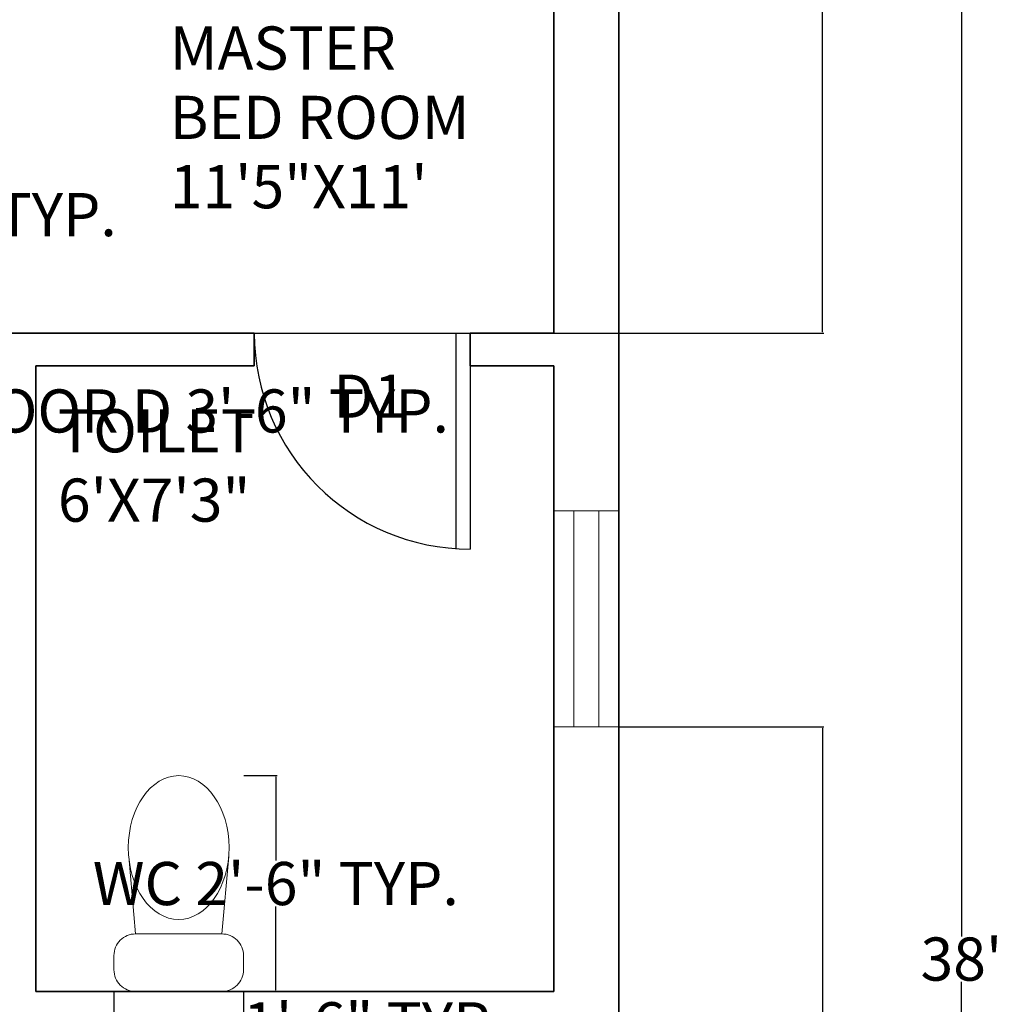
# Model space of a CAD drawing. Units: inches. Extents: x -26 to 575, y -18 to 513.
# Tile 27 of 28: x 439 to 575, y 241 to 378. Entities that reach past the tile are written whole.
import ezdxf

# ---------------------------------------------------------------- set-up
doc = ezdxf.new("R2010")
doc.units = ezdxf.units.IN
doc.header["$MEASUREMENT"] = 0
for name, color, linetype, lineweight in [('A-ANNO-DIMS', 2, 'Continuous', 18), ('A-ANNO-TEXT', 7, 'Continuous', 18), ('A-AREA-IDEN', 7, 'Continuous', 18), ('A-DOOR', 3, 'Continuous', 25), ('A-FLOR-FIXT', 9, 'Continuous', 18), ('A-GLAZ', 4, 'Continuous', 18), ('A-WALL', 7, 'Continuous', 35)]:
    doc.layers.add(name, color=color, linetype=linetype, lineweight=lineweight)
doc.styles.get("Standard").update_dxf_attribs({"font": 'arial.ttf', "height": 6})
doc.dimstyles.get("Standard").update_dxf_attribs({"dimtxt": 6, "dimasz": 0.18, "dimexe": 0.18, "dimexo": 0.0625, "dimgap": 0.09, "dimtad": 0, "dimtih": 1, "dimtoh": 1, "dimzin": 0, "dimdsep": 46, "dimlunit": 3, "dimtxsty": 'Standard', "dimcen": 0.09, "dimadec": 0, "dimazin": 0, "dimtfac": 1, "dimtofl": 0, "dimtmove": 0, "dimatfit": 3, "dimfxl": 1, "dimtolj": 1, "dimtzin": 0, "dimarcsym": 0})

# ---------------------------------------------------------------- blocks, each defined once
blk = doc.blocks.new('*D2')
at = {"layer": 'A-ANNO-DIMS', "color": 0, "lineweight": -2, "transparency": 16777216}
for p, q in [((522.24, 475.51), (569.98, 475.51)), ((569.8, 475.33), (569.8, 250.66)), ((569.8, 19.69), (569.8, 244.35)), ((522.24, 19.51), (569.98, 19.51))]:
    blk.add_line(p, q, dxfattribs=at)
at = {"layer": 'A-ANNO-DIMS', "color": 0, "transparency": 16777216}
for points in [[(569.77, 475.33), (569.83, 475.33), (569.8, 475.51)], [(569.77, 19.69), (569.83, 19.69), (569.8, 19.51)]]:
    blk.add_solid(points, dxfattribs=at)
at = {"layer": 'Defpoints', "color": 0, "transparency": 16777216}
for p in [(522.18, 475.51), (522.18, 19.51), (569.8, 19.51)]:
    blk.add_point(p, dxfattribs=at)
at = {"layer": 'A-ANNO-DIMS', "color": 0, "transparency": 16777216, "insert": (569.8, 247.51), "char_height": 6, "attachment_point": 5}
blk.add_mtext("\\A1;38'", dxfattribs=at)
blk = doc.blocks.new('DOOR-SWING-30IN')
for p, q in [((-30, 0), (0, 0)), ((-2, 0), (-2, -30)), ((0, 0), (0, -30))]:
    blk.add_line(p, q)
blk.add_arc((0, 0), 30, 180, 270)
blk = doc.blocks.new('WINDOW-30IN')
for p, q in [((30, 9), (0, 9)), ((0, 9), (0, 0)), ((30, 0), (30, 9)), ((30, 6.25), (0, 6.25)), ((30, 0), (30, 4.5)), ((30, 2.75), (0, 2.75)), ((0, 0), (30, 0))]:
    blk.add_line(p, q)
blk = doc.blocks.new('WC-FLOOR-MOUNT')
for p, q in [((-6, 8), (-6.95, 18.75)), ((6, 8), (6.95, 18.75))]:
    blk.add_line(p, q)
blk.add_lwpolyline([(-6, 8), (6, 8, -0.414214), (9, 5), (9, 3, -0.414214), (6, 0), (-6, 0, -0.414214), (-9, 3), (-9, 5, -0.414214)], format="xyb", close=True)
blk.add_ellipse((0, 20), major_axis=(0, 10), ratio=0.7)
blk = doc.blocks.new('*D14')
at = {"layer": 'A-ANNO-DIMS', "color": 0, "lineweight": -2, "transparency": 16777216}
for p, q in [((385.8, 329.95), (385.8, 323.53)), ((427.8, 329.95), (427.8, 323.53)), ((385.98, 323.71), (427.62, 323.71)), ((427.8, 323.71), (427.98, 323.71))]:
    blk.add_line(p, q, dxfattribs=at)
at = {"layer": 'A-ANNO-DIMS', "color": 0, "transparency": 16777216}
for points in [[(385.98, 323.74), (385.98, 323.68), (385.8, 323.71)], [(427.62, 323.74), (427.62, 323.68), (427.8, 323.71)]]:
    blk.add_solid(points, dxfattribs=at)
at = {"layer": 'Defpoints', "color": 0, "transparency": 16777216}
for p in [(385.8, 330.01), (427.8, 330.01), (427.8, 323.71)]:
    blk.add_point(p, dxfattribs=at)
at = {"layer": 'A-ANNO-DIMS', "color": 0, "transparency": 16777216, "insert": (464.13, 323.71), "char_height": 6, "attachment_point": 5}
blk.add_mtext('\\A1;DOOR D 3\'-6" TYP.', dxfattribs=at)
blk = doc.blocks.new('*D15')
at = {"layer": 'A-ANNO-DIMS', "color": 0, "lineweight": -2, "transparency": 16777216}
for p, q in [((427.86, 372.01), (434.28, 372.01)), ((434.1, 371.83), (434.1, 354.16)), ((434.1, 330.19), (434.1, 347.85)), ((427.86, 330.01), (434.28, 330.01))]:
    blk.add_line(p, q, dxfattribs=at)
at = {"layer": 'A-ANNO-DIMS', "color": 0, "transparency": 16777216}
for points in [[(434.07, 371.83), (434.13, 371.83), (434.1, 372.01)], [(434.07, 330.19), (434.13, 330.19), (434.1, 330.01)]]:
    blk.add_solid(points, dxfattribs=at)
at = {"layer": 'Defpoints', "color": 0, "transparency": 16777216}
for p in [(427.8, 372.01), (434.1, 372.01), (427.8, 330.01)]:
    blk.add_point(p, dxfattribs=at)
at = {"layer": 'A-ANNO-DIMS', "color": 0, "transparency": 16777216, "insert": (434.1, 351.01), "char_height": 6, "attachment_point": 5}
blk.add_mtext('\\A1;3\'-6" TYP.', dxfattribs=at)
blk = doc.blocks.new('*D20')
at = {"layer": 'A-ANNO-DIMS', "color": 0, "lineweight": -2, "transparency": 16777216}
for p, q in [((470.08, 273.01), (474.7, 273.01)), ((474.52, 272.83), (474.52, 261.2)), ((474.52, 243.19), (474.52, 254.82)), ((470.08, 243.01), (474.7, 243.01))]:
    blk.add_line(p, q, dxfattribs=at)
at = {"layer": 'A-ANNO-DIMS', "color": 0, "transparency": 16777216}
for points in [[(474.49, 272.83), (474.55, 272.83), (474.52, 273.01)], [(474.49, 243.19), (474.55, 243.19), (474.52, 243.01)]]:
    blk.add_solid(points, dxfattribs=at)
at = {"layer": 'Defpoints', "color": 0, "transparency": 16777216}
for p in [(470.02, 273.01), (474.52, 273.01), (470.02, 243.01)]:
    blk.add_point(p, dxfattribs=at)
at = {"layer": 'A-ANNO-DIMS', "color": 0, "transparency": 16777216, "insert": (474.52, 258.01), "char_height": 6, "attachment_point": 5}
blk.add_mtext('\\A1;WC 2\'-6" TYP.', dxfattribs=at)
blk = doc.blocks.new('*D21')
at = {"layer": 'A-ANNO-DIMS', "color": 0, "lineweight": -2, "transparency": 16777216}
for p, q in [((452.02, 242.95), (452.02, 238.33)), ((470.02, 242.95), (470.02, 238.33)), ((452.2, 238.51), (469.84, 238.51)), ((470.02, 238.51), (470.2, 238.51))]:
    blk.add_line(p, q, dxfattribs=at)
at = {"layer": 'A-ANNO-DIMS', "color": 0, "transparency": 16777216}
for points in [[(452.2, 238.54), (452.2, 238.48), (452.02, 238.51)], [(469.84, 238.54), (469.84, 238.48), (470.02, 238.51)]]:
    blk.add_solid(points, dxfattribs=at)
at = {"layer": 'Defpoints', "color": 0, "transparency": 16777216}
for p in [(452.02, 243.01), (470.02, 243.01), (470.02, 238.51)]:
    blk.add_point(p, dxfattribs=at)
at = {"layer": 'A-ANNO-DIMS', "color": 0, "transparency": 16777216, "insert": (488.3, 238.51), "char_height": 6, "attachment_point": 5}
blk.add_mtext('\\A1;1\'-6" TYP.', dxfattribs=at)
blk = doc.blocks.new('*D43')
at = {"layer": 'A-ANNO-DIMS', "color": 0, "lineweight": -2, "transparency": 16777216}
for p, q in [((522.24, 279.8), (550.66, 279.8)), ((550.48, 279.62), (550.48, 239.53)), ((550.48, 193.11), (550.48, 233.21)), ((522.24, 192.93), (550.66, 192.93))]:
    blk.add_line(p, q, dxfattribs=at)
at = {"layer": 'A-ANNO-DIMS', "color": 0, "transparency": 16777216}
for points in [[(550.45, 279.62), (550.51, 279.62), (550.48, 279.8)], [(550.45, 193.11), (550.51, 193.11), (550.48, 192.93)]]:
    blk.add_solid(points, dxfattribs=at)
at = {"layer": 'Defpoints', "color": 0, "transparency": 16777216}
for p in [(522.18, 279.8), (550.48, 279.8), (522.18, 192.93)]:
    blk.add_point(p, dxfattribs=at)
at = {"layer": 'A-ANNO-DIMS', "color": 0, "transparency": 16777216, "insert": (550.48, 236.37), "char_height": 6, "attachment_point": 5}
blk.add_mtext('\\A1;7\'-3"', dxfattribs=at)
blk = doc.blocks.new('*D49')
at = {"layer": 'A-ANNO-DIMS', "color": 0, "lineweight": -2, "transparency": 16777216}
for p, q in [((278.24, 466.51), (550.66, 466.51)), ((550.48, 466.33), (550.48, 403.66)), ((550.48, 334.69), (550.48, 397.35)), ((278.24, 334.51), (550.66, 334.51))]:
    blk.add_line(p, q, dxfattribs=at)
at = {"layer": 'A-ANNO-DIMS', "color": 0, "transparency": 16777216}
for points in [[(550.45, 466.33), (550.51, 466.33), (550.48, 466.51)], [(550.45, 334.69), (550.51, 334.69), (550.48, 334.51)]]:
    blk.add_solid(points, dxfattribs=at)
at = {"layer": 'Defpoints', "color": 0, "transparency": 16777216}
for p in [(278.18, 466.51), (550.48, 466.51), (278.18, 334.51)]:
    blk.add_point(p, dxfattribs=at)
at = {"layer": 'A-ANNO-DIMS', "color": 0, "transparency": 16777216, "insert": (550.48, 400.51), "char_height": 6, "attachment_point": 5}
blk.add_mtext('\\A1;11\'-0"', dxfattribs=at)

msp = doc.modelspace()

# ---------------------------------------------------------------- linework, layer by layer
at = {"layer": 'A-WALL'}
for p, q in [((513.177, 334.508), (513.177, 466.508)), ((471.534, 334.508), (427.797, 334.508)), ((471.534, 330.008), (471.534, 334.508)), ((513.177, 334.508), (501.534, 334.508)), ((501.534, 330.008), (501.534, 334.508)), ((441.177, 243.008), (441.177, 330.008)), ((471.534, 330.008), (441.177, 330.008)), ((513.177, 330.008), (501.534, 330.008)), ((513.177, 243.008), (513.177, 330.008)), ((513.177, 243.008), (441.177, 243.008))]:
    msp.add_line(p, q, dxfattribs=at)
msp.add_lwpolyline([(18.177, 19.508), (522.177, 19.508), (522.177, 475.508), (18.177, 475.508)], close=True, dxfattribs=at)

# ---------------------------------------------------------------- block references
at = {"layer": 'A-DOOR'}
msp.add_blockref('DOOR-SWING-30IN', (501.534, 334.508), dxfattribs=at)
at = {"layer": 'A-FLOR-FIXT'}
msp.add_blockref('WC-FLOOR-MOUNT', (461.022, 243.008), dxfattribs=at)
at = {"layer": 'A-GLAZ', "extrusion": (0, 0, -1), "zscale": -1, "rotation": 89.99999999999967}
msp.add_blockref('WINDOW-30IN', (-513.177, 279.805), dxfattribs=at)

# ---------------------------------------------------------------- texts
at = {"layer": 'A-ANNO-TEXT'}
msp.add_text('D1', height=6, rotation=0.00167, dxfattribs=at).set_placement((482.498, 322.767))
at = {"layer": 'A-AREA-IDEN'}
for s, p in [('MASTER', (459.779, 371.165)), ('BED ROOM', (459.78, 361.527)), ('11\'5"X11\'', (459.78, 351.888)), ('TOILET', (444.238, 317.953)), ('6\'X7\'3"', (444.239, 308.315))]:
    msp.add_text(s, height=6, rotation=0.00167, dxfattribs=at).set_placement(p)

# ---------------------------------------------------------------- dimensions: what is measured, and where the dimension line sits
at = {"layer": 'A-ANNO-DIMS'}
for base, p1, p2, override, picture, middle in [((569.801, 19.508), (522.177, 475.508), (522.177, 19.508), {"dimclrd": 0, "dimclre": 0, "dimclrt": 0}, '*D2', (569.801, 247.508)), ((550.477, 466.508), (278.177, 334.508), (278.177, 466.508), {"dimdec": 1, "dimlfac": 1, "dimrnd": 0, "dimzin": 1, "dimdsep": 46, "dimlunit": 4, "dimfrac": 2}, '*D49', (550.477, 400.508)), ((550.477, 279.805), (522.177, 192.934), (522.177, 279.805), {"dimdec": 1, "dimlfac": 1, "dimrnd": 0, "dimzin": 1, "dimdsep": 46, "dimlunit": 4, "dimfrac": 2}, '*D43', (550.477, 236.37))]:
    dim = msp.add_linear_dim(base=base, p1=p1, p2=p2, angle=90, dimstyle='Standard', override=override, dxfattribs=at)
    dim.commit()
    dim.dimension.update_dxf_attribs({"geometry": picture, "text_midpoint": middle})
for base, p1, p2, text, picture, middle in [((434.097, 372.008), (427.797, 330.008), (427.797, 372.008), '<> TYP.', '*D15', (434.097, 351.008)), ((474.522, 273.008), (470.022, 243.008), (470.022, 273.008), 'WC <> TYP.', '*D20', (474.522, 258.008))]:
    dim = msp.add_linear_dim(base=base, p1=p1, p2=p2, angle=90, text=text, dimstyle='Standard', override={"dimdec": 1, "dimlfac": 1, "dimrnd": 0, "dimzin": 1, "dimdsep": 46, "dimlunit": 4, "dimfrac": 2}, dxfattribs=at)
    dim.commit()
    dim.dimension.update_dxf_attribs({"geometry": picture, "text_midpoint": middle})
for base, p1, p2, text, picture, middle in [((427.797, 323.708), (385.797, 330.008), (427.797, 330.008), 'DOOR D <> TYP.', '*D14', (464.132, 323.708)), ((470.022, 238.508), (452.022, 243.008), (470.022, 243.008), '<> TYP.', '*D21', (488.297, 238.508))]:
    dim = msp.add_linear_dim(base=base, p1=p1, p2=p2, text=text, dimstyle='Standard', override={"dimdec": 1, "dimlfac": 1, "dimrnd": 0, "dimzin": 1, "dimdsep": 46, "dimlunit": 4, "dimfrac": 2}, dxfattribs=at)
    dim.commit()
    dim.dimension.update_dxf_attribs({"geometry": picture, "text_midpoint": middle})

doc.saveas('drawing.dxf')
